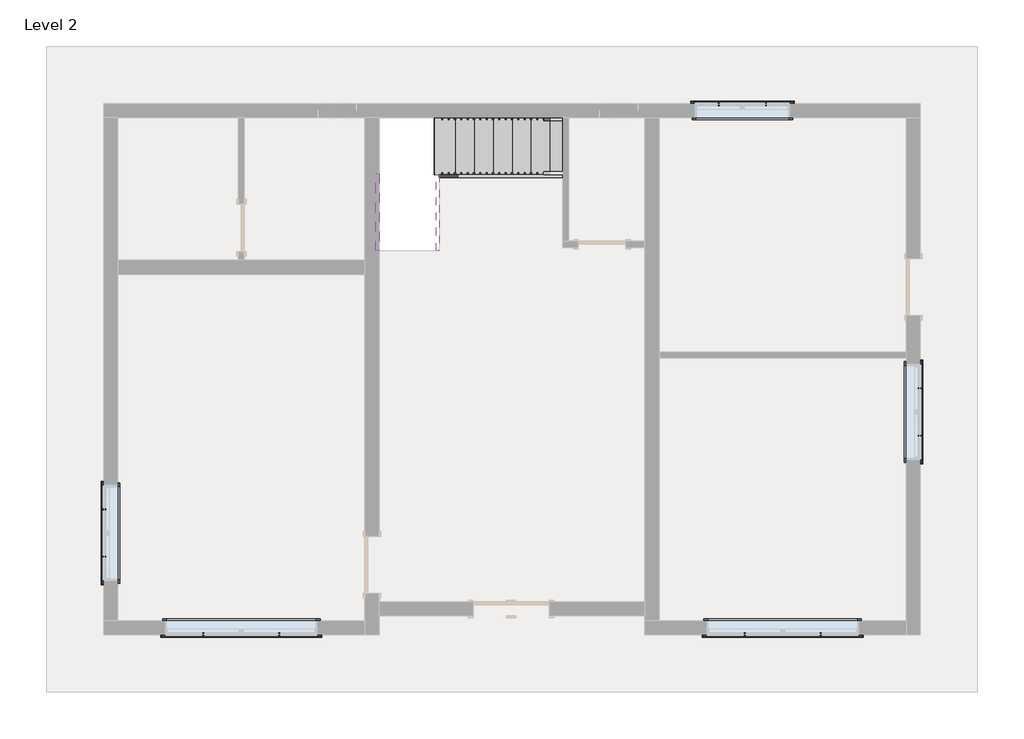
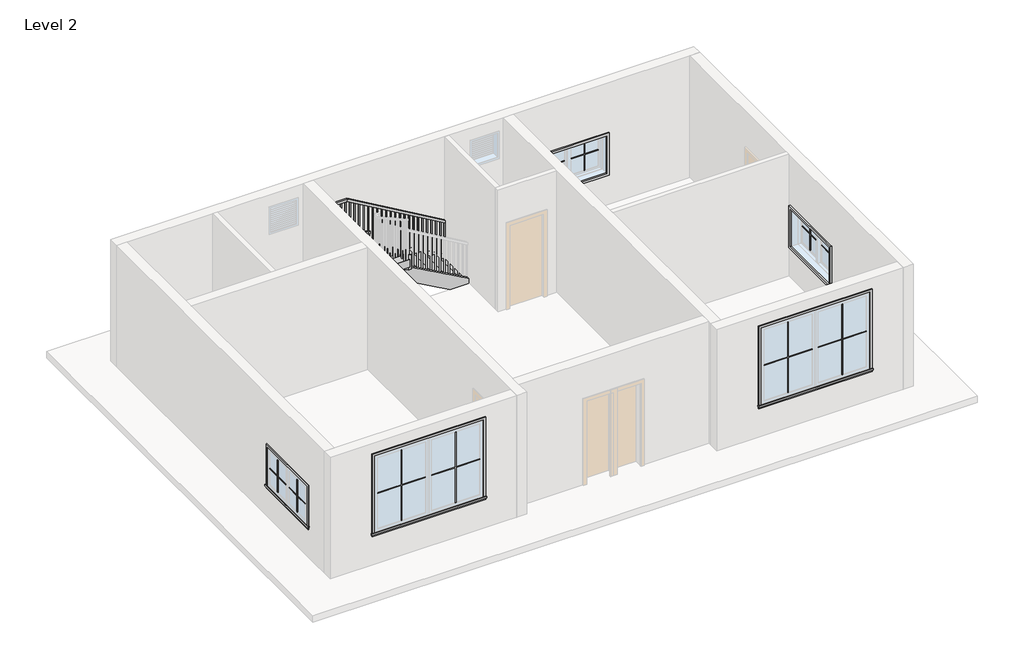
# One storey, part 2 of 2: 20 proxies, 4 members, 1 railing, 1 stair flight.
"""IFC4 building model written with IfcOpenShell, lengths in millimetres."""

from ifc_helpers import new_model, si_unit, frame, origin, place, context, project, spatial, polyline, outline, extrude, faceted_brep, transform, mapped, element, save
from components import muntin_pattern_2x2_muntin_pattern_2x2_9352d081, muntin_pattern_2x2_muntin_pattern_2x2_5c2cbe28, muntin_pattern_2x2_muntin_pattern_2x2_bb8d4d84, muntin_pattern_2x2_muntin_pattern_2x2_d03a1f3c, trim_window_exterior_flat_with_sill_979bde60, trim_window_exterior_flat_with_sill_359ed2ce, trim_window_interior_flat_picture_frame_7883d11b, trim_window_interior_flat_picture_frame_939a8053, stair_flight_cf719367

model = new_model("IFC4")

# Units and contexts
model_context = context("Model", 3, world=origin())
ifc_project = project(units=[si_unit("LENGTHUNIT", "METRE", prefix="MILLI")], contexts=[model_context])

# Site, building, storey
site = spatial("IfcSite", under=ifc_project)
building = spatial("IfcBuilding", under=site)
storey = spatial("IfcBuildingStorey", under=building, Name="Level 2", Elevation=3048.0)

# Proxies
placement = place(None, origin())
muntin_pattern_2x2_muntin_pattern_2x2_shape = muntin_pattern_2x2_muntin_pattern_2x2_9352d081(model_context)
element("IfcBuildingElementProxy", 1, Name="Muntin Pattern_2x2 : Muntin Pattern_2x2", ObjectType="Muntin Pattern_2x2 : Muntin Pattern_2x2", at=placement, inside=storey, context=model_context, shape_type="MappedRepresentation", body=[
    mapped(muntin_pattern_2x2_muntin_pattern_2x2_shape, transform((-7798.9165084, -1764.5743005, 4032.25), x_axis=(0.0, 1.0, 0.0), y_axis=(-1.0, 0.0, 0.0), z_axis=(0.0, 0.0, 1.0))),
])
element("IfcBuildingElementProxy", 2, Name="Muntin Pattern_2x2 : Muntin Pattern_2x2", ObjectType="Muntin Pattern_2x2 : Muntin Pattern_2x2", at=placement, inside=storey, context=model_context, shape_type="MappedRepresentation", body=[
    mapped(muntin_pattern_2x2_muntin_pattern_2x2_shape, transform((5288.4334916, 937.3506995, 4032.25), x_axis=(0.0, -1.0, 0.0), y_axis=(1.0, 0.0, 0.0), z_axis=(0.0, 0.0, 1.0))),
])
element("IfcBuildingElementProxy", 3, Name="Muntin Pattern_2x2 : Muntin Pattern_2x2", ObjectType="Muntin Pattern_2x2 : Muntin Pattern_2x2", at=placement, inside=storey, context=model_context, shape_type="MappedRepresentation", body=[
    mapped(muntin_pattern_2x2_muntin_pattern_2x2_shape, transform((2061.0459916, 5501.4131995, 4032.25), x_axis=(1.0, 0.0, 0.0), y_axis=(0.0, 1.0, 0.0), z_axis=(0.0, 0.0, 1.0))),
])
muntin_pattern_2x2_muntin_pattern_2x2_2_shape = muntin_pattern_2x2_muntin_pattern_2x2_5c2cbe28(model_context)
element("IfcBuildingElementProxy", 4, Name="Muntin Pattern_2x2 : Muntin Pattern_2x2", ObjectType="Muntin Pattern_2x2 : Muntin Pattern_2x2", at=placement, inside=storey, context=model_context, shape_type="MappedRepresentation", body=[
    mapped(muntin_pattern_2x2_muntin_pattern_2x2_2_shape, transform((-7798.9165084, -1005.7493005, 4032.25), x_axis=(0.0, -1.0, 0.0), y_axis=(1.0, 0.0, 0.0), z_axis=(0.0, 0.0, 1.0))),
])
element("IfcBuildingElementProxy", 5, Name="Muntin Pattern_2x2 : Muntin Pattern_2x2", ObjectType="Muntin Pattern_2x2 : Muntin Pattern_2x2", at=placement, inside=storey, context=model_context, shape_type="MappedRepresentation", body=[
    mapped(muntin_pattern_2x2_muntin_pattern_2x2_2_shape, transform((5288.4334916, 178.5256995, 4032.25), x_axis=(0.0, 1.0, 0.0), y_axis=(-1.0, 0.0, 0.0), z_axis=(0.0, 0.0, 1.0))),
])
element("IfcBuildingElementProxy", 6, Name="Muntin Pattern_2x2 : Muntin Pattern_2x2", ObjectType="Muntin Pattern_2x2 : Muntin Pattern_2x2", at=placement, inside=storey, context=model_context, shape_type="MappedRepresentation", body=[
    mapped(muntin_pattern_2x2_muntin_pattern_2x2_2_shape, transform((2819.8709916, 5501.4131995, 4032.25), x_axis=(-1.0, 0.0, 0.0), y_axis=(0.0, -1.0, 0.0), z_axis=(0.0, 0.0, 1.0))),
])
muntin_pattern_2x2_muntin_pattern_2x2_3_shape = muntin_pattern_2x2_muntin_pattern_2x2_bb8d4d84(model_context)
element("IfcBuildingElementProxy", 7, Name="Muntin Pattern_2x2 : Muntin Pattern_2x2", ObjectType="Muntin Pattern_2x2 : Muntin Pattern_2x2", at=placement, inside=storey, context=model_context, shape_type="MappedRepresentation", body=[
    mapped(muntin_pattern_2x2_muntin_pattern_2x2_3_shape, transform((-4990.6290084, -3013.9368005, 4032.25), x_axis=(-1.0, 0.0, 0.0), y_axis=(0.0, -1.0, 0.0), z_axis=(0.0, 0.0, 1.0))),
])
element("IfcBuildingElementProxy", 8, Name="Muntin Pattern_2x2 : Muntin Pattern_2x2", ObjectType="Muntin Pattern_2x2 : Muntin Pattern_2x2", at=placement, inside=storey, context=model_context, shape_type="MappedRepresentation", body=[
    mapped(muntin_pattern_2x2_muntin_pattern_2x2_3_shape, transform((3696.1709916, -3013.9368005, 4032.25), x_axis=(-1.0, 0.0, 0.0), y_axis=(0.0, -1.0, 0.0), z_axis=(0.0, 0.0, 1.0))),
])
muntin_pattern_2x2_muntin_pattern_2x2_4_shape = muntin_pattern_2x2_muntin_pattern_2x2_d03a1f3c(model_context)
element("IfcBuildingElementProxy", 9, Name="Muntin Pattern_2x2 : Muntin Pattern_2x2", ObjectType="Muntin Pattern_2x2 : Muntin Pattern_2x2", at=placement, inside=storey, context=model_context, shape_type="MappedRepresentation", body=[
    mapped(muntin_pattern_2x2_muntin_pattern_2x2_4_shape, transform((-6206.6540084, -3013.9368005, 4032.25), x_axis=(1.0, 0.0, 0.0), y_axis=(0.0, 1.0, 0.0), z_axis=(0.0, 0.0, 1.0))),
])
element("IfcBuildingElementProxy", 10, Name="Muntin Pattern_2x2 : Muntin Pattern_2x2", ObjectType="Muntin Pattern_2x2 : Muntin Pattern_2x2", at=placement, inside=storey, context=model_context, shape_type="MappedRepresentation", body=[
    mapped(muntin_pattern_2x2_muntin_pattern_2x2_4_shape, transform((2480.1459916, -3013.9368005, 4032.25), x_axis=(1.0, 0.0, 0.0), y_axis=(0.0, 1.0, 0.0), z_axis=(0.0, 0.0, 1.0))),
])
trim_window_exterior_flat_with_sill_shape = trim_window_exterior_flat_with_sill_979bde60(model_context)
element("IfcBuildingElementProxy", 11, Name="Trim-Window-Exterior-Flat : with Sill", ObjectType="Trim-Window-Exterior-Flat : with Sill", at=placement, inside=storey, context=model_context, shape_type="MappedRepresentation", body=[
    mapped(trim_window_exterior_flat_with_sill_shape, transform((-7808.4415084, -1385.1618005, 4876.8), x_axis=(0.0, -1.0, 0.0), y_axis=(0.0, 0.0, 1.0), z_axis=(-1.0, 0.0, 0.0))),
])
element("IfcBuildingElementProxy", 12, Name="Trim-Window-Exterior-Flat : with Sill", ObjectType="Trim-Window-Exterior-Flat : with Sill", at=placement, inside=storey, context=model_context, shape_type="MappedRepresentation", body=[
    mapped(trim_window_exterior_flat_with_sill_shape, transform((5297.9584916, 557.9381995, 4876.8), x_axis=(0.0, 1.0, 0.0), y_axis=(0.0, 0.0, 1.0), z_axis=(1.0, 0.0, 0.0))),
])
element("IfcBuildingElementProxy", 13, Name="Trim-Window-Exterior-Flat : with Sill", ObjectType="Trim-Window-Exterior-Flat : with Sill", at=placement, inside=storey, context=model_context, shape_type="MappedRepresentation", body=[
    mapped(trim_window_exterior_flat_with_sill_shape, transform((2440.4584916, 5510.9381995, 4876.8), x_axis=(-1.0, 0.0, 0.0), y_axis=(0.0, 0.0, 1.0), z_axis=(0.0, 1.0, 0.0))),
])
trim_window_exterior_flat_with_sill_2_shape = trim_window_exterior_flat_with_sill_359ed2ce(model_context)
element("IfcBuildingElementProxy", 14, Name="Trim-Window-Exterior-Flat : with Sill", ObjectType="Trim-Window-Exterior-Flat : with Sill", at=placement, inside=storey, context=model_context, shape_type="MappedRepresentation", body=[
    mapped(trim_window_exterior_flat_with_sill_2_shape, transform((-5598.6415084, -3023.4618005, 5791.2), x_axis=(1.0, 0.0, 0.0), y_axis=(0.0, 0.0, 1.0), z_axis=(0.0, -1.0, 0.0))),
])
element("IfcBuildingElementProxy", 15, Name="Trim-Window-Exterior-Flat : with Sill", ObjectType="Trim-Window-Exterior-Flat : with Sill", at=placement, inside=storey, context=model_context, shape_type="MappedRepresentation", body=[
    mapped(trim_window_exterior_flat_with_sill_2_shape, transform((3088.1584916, -3023.4618005, 5791.2), x_axis=(1.0, 0.0, 0.0), y_axis=(0.0, 0.0, 1.0), z_axis=(0.0, -1.0, 0.0))),
])
trim_window_interior_flat_picture_frame_shape = trim_window_interior_flat_picture_frame_7883d11b(model_context)
element("IfcBuildingElementProxy", 16, Name="Trim-Window-Interior-Flat : Picture Frame", ObjectType="Trim-Window-Interior-Flat : Picture Frame", at=placement, inside=storey, context=model_context, shape_type="MappedRepresentation", body=[
    mapped(trim_window_interior_flat_picture_frame_shape, transform((-7579.8415084, -1385.1618005, 4876.8), x_axis=(0.0, 1.0, 0.0), y_axis=(0.0, 0.0, 1.0), z_axis=(1.0, 0.0, 0.0))),
])
element("IfcBuildingElementProxy", 17, Name="Trim-Window-Interior-Flat : Picture Frame", ObjectType="Trim-Window-Interior-Flat : Picture Frame", at=placement, inside=storey, context=model_context, shape_type="MappedRepresentation", body=[
    mapped(trim_window_interior_flat_picture_frame_shape, transform((5069.3584916, 557.9381995, 4876.8), x_axis=(0.0, -1.0, 0.0), y_axis=(0.0, 0.0, 1.0), z_axis=(-1.0, 0.0, 0.0))),
])
element("IfcBuildingElementProxy", 18, Name="Trim-Window-Interior-Flat : Picture Frame", ObjectType="Trim-Window-Interior-Flat : Picture Frame", at=placement, inside=storey, context=model_context, shape_type="MappedRepresentation", body=[
    mapped(trim_window_interior_flat_picture_frame_shape, transform((2440.4584916, 5282.3381995, 4876.8), x_axis=(1.0, 0.0, 0.0), y_axis=(0.0, 0.0, 1.0), z_axis=(0.0, -1.0, 0.0))),
])
trim_window_interior_flat_picture_frame_2_shape = trim_window_interior_flat_picture_frame_939a8053(model_context)
element("IfcBuildingElementProxy", 19, Name="Trim-Window-Interior-Flat : Picture Frame", ObjectType="Trim-Window-Interior-Flat : Picture Frame", at=placement, inside=storey, context=model_context, shape_type="MappedRepresentation", body=[
    mapped(trim_window_interior_flat_picture_frame_2_shape, transform((-5598.6415084, -2794.8618005, 5791.2), x_axis=(-1.0, 0.0, 0.0), y_axis=(0.0, 0.0, 1.0), z_axis=(0.0, 1.0, 0.0))),
])
element("IfcBuildingElementProxy", 20, Name="Trim-Window-Interior-Flat : Picture Frame", ObjectType="Trim-Window-Interior-Flat : Picture Frame", at=placement, inside=storey, context=model_context, shape_type="MappedRepresentation", body=[
    mapped(trim_window_interior_flat_picture_frame_2_shape, transform((3088.1584916, -2794.8618005, 5791.2), x_axis=(-1.0, 0.0, 0.0), y_axis=(0.0, 0.0, 1.0), z_axis=(0.0, 1.0, 0.0))),
])

# Members
element("IfcMember", 21, ObjectType="Stringer - 2\" Width", at=placement, inside=storey, context=model_context, shape_type="SweptSolid", body=[
    extrude(outline(polyline([(3048.0, -442.4415084), (3312.0428392, -442.4415084), (4412.7095059, -2423.6415084), (4064.0308318, -2423.6415084), (3048.0, -594.7860112), (3048.0, -442.4415084)])), frame((0.0, 4317.5146777, 0.0), z_axis=(0.0, 1.0, 0.0), x_axis=(0.0, 0.0, 1.0)), (0.0, 0.0, 1.0), 50.8),
])
element("IfcMember", 22, ObjectType="Stringer - 2\" Width", at=placement, inside=storey, context=model_context, shape_type="SweptSolid", body=[
    extrude(outline(polyline([(4368.3146777, 4610.245537), (4368.3146777, 4261.6006925), (3148.7383287, 4938.8643411), (3148.7383287, 5287.5091856), (4368.3146777, 4610.245537)])), frame((-2474.4415084, 0.0, 0.0), z_axis=(1.0, 0.0, 0.0), x_axis=(0.0, 1.0, 0.0)), (0.0, 0.0, 1.0), 50.8),
])
element("IfcMember", 23, ObjectType="Stringer - 2\" Width", at=placement, inside=storey, context=model_context, shape_type="SweptSolid", body=[
    extrude(outline(polyline([(3048.0, -442.4415084), (3312.0428392, -442.4415084), (4102.6636166, -1865.5589077), (4102.6636166, -2493.1805211), (3048.0, -594.7860112), (3048.0, -442.4415084)])), frame((0.0, 5282.3381995, 0.0), z_axis=(0.0, 1.0, 0.0), x_axis=(0.0, 0.0, 1.0)), (0.0, 0.0, 1.0), 50.8),
])
element("IfcMember", 24, ObjectType="Stringer - 2\" Width", at=placement, inside=storey, context=model_context, shape_type="SweptSolid", body=[
    extrude(outline(polyline([(3758.489521, 4600.253054), (3148.7383287, 4938.8643411), (3148.7383287, 5287.5091856), (4386.3085505, 4600.253054), (3758.489521, 4600.253054)])), frame((-3439.6415084, 0.0, 0.0), z_axis=(1.0, 0.0, 0.0), x_axis=(0.0, 1.0, 0.0)), (0.0, 0.0, 1.0), 50.8),
])

# Railing
element("IfcRailing", 25, ObjectType="Handrail - Rectangular", at=placement, inside=storey, context=model_context, shape_type="SolidModel", body=[
    faceted_brep([(-442.4415084, 5231.5381995, 4131.7333333), (-442.4415084, 5231.5381995, 4072.9219871), (-442.4415084, 5282.3381995, 4072.9219871), (-442.4415084, 5282.3381995, 4131.7333333), (-2641.0608886, 5231.5381995, 5414.2613051), (-2654.794625, 5231.5381995, 5363.4613051), (-2654.794625, 5282.3381995, 5363.4613051), (-2641.0608886, 5282.3381995, 5414.2613051), (-3338.0415084, 5231.5381995, 5414.2613051), (-3338.0415084, 5231.5381995, 5363.4613051), (-3388.8415084, 5282.3381995, 5363.4613051), (-3388.8415084, 5282.3381995, 5414.2613051), (-3338.0415084, 4498.2044111, 5414.2613051), (-3338.0415084, 4485.04436, 5363.4613051), (-3388.8415084, 4485.04436, 5363.4613051), (-3388.8415084, 4498.2044111, 5414.2613051), (-3338.0415084, 3148.7383287, 6163.7333333), (-3388.8415084, 3148.7383287, 6163.7333333), (-3388.8415084, 3148.7383287, 6105.62445), (-3338.0415084, 3148.7383287, 6105.62445)], [[[0, 1, 2, 3]], [[1, 0, 4, 5]], [[2, 1, 5, 6]], [[3, 2, 6, 7]], [[0, 3, 7, 4]], [[5, 4, 8, 9]], [[6, 5, 9, 10]], [[7, 6, 10, 11]], [[4, 7, 11, 8]], [[9, 8, 12, 13]], [[10, 9, 13, 14]], [[11, 10, 14, 15]], [[8, 11, 15, 12]], [[16, 17, 18, 19]], [[13, 12, 16, 19]], [[14, 13, 19, 18]], [[15, 14, 18, 17]], [[12, 15, 17, 16]]]),
    extrude(outline(polyline([(3215.4131995, 6068.5942858), (3234.4631995, 6058.0142183), (3234.4631995, 5080.0), (3215.4131995, 5080.0), (3215.4131995, 6068.5942858)])), frame((-3372.9665084, 0.0, 0.0), z_axis=(1.0, 0.0, 0.0), x_axis=(0.0, 1.0, 0.0)), (0.0, 0.0, 1.0), 19.05),
    extrude(outline(polyline([(3317.0131995, 6012.3240232), (3336.0631995, 6001.7439558), (3336.0631995, 5080.0), (3317.0131995, 5080.0), (3317.0131995, 6012.3240232)])), frame((-3372.9665084, 0.0, 0.0), z_axis=(1.0, 0.0, 0.0), x_axis=(0.0, 1.0, 0.0)), (0.0, 0.0, 1.0), 19.05),
    extrude(outline(polyline([(3418.6131995, 5955.8969969), (3437.6631995, 5945.3169295), (3437.6631995, 5080.0), (3418.6131995, 5080.0), (3418.6131995, 5955.8969969)])), frame((-3372.9665084, 0.0, 0.0), z_axis=(1.0, 0.0, 0.0), x_axis=(0.0, 1.0, 0.0)), (0.0, 0.0, 1.0), 19.05),
    extrude(outline(polyline([(3520.2131995, 5899.4699707), (3539.2631995, 5888.8899033), (3539.2631995, 4910.6666667), (3520.2131995, 4910.6666667), (3520.2131995, 5899.4699707)])), frame((-3372.9665084, 0.0, 0.0), z_axis=(1.0, 0.0, 0.0), x_axis=(0.0, 1.0, 0.0)), (0.0, 0.0, 1.0), 19.05),
    extrude(outline(polyline([(3621.8131995, 5842.9906899), (3640.8631995, 5832.4106224), (3640.8631995, 4910.6666667), (3621.8131995, 4910.6666667), (3621.8131995, 5842.9906899)])), frame((-3372.9665084, 0.0, 0.0), z_axis=(1.0, 0.0, 0.0), x_axis=(0.0, 1.0, 0.0)), (0.0, 0.0, 1.0), 19.05),
    extrude(outline(polyline([(3723.4131995, 5786.5636636), (3742.4631995, 5775.9835962), (3742.4631995, 4910.6666667), (3723.4131995, 4910.6666667), (3723.4131995, 5786.5636636)])), frame((-3372.9665084, 0.0, 0.0), z_axis=(1.0, 0.0, 0.0), x_axis=(0.0, 1.0, 0.0)), (0.0, 0.0, 1.0), 19.05),
    extrude(outline(polyline([(3825.0131995, 5730.1366374), (3844.0631995, 5719.5565699), (3844.0631995, 4741.3333333), (3825.0131995, 4741.3333333), (3825.0131995, 5730.1366374)])), frame((-3372.9665084, 0.0, 0.0), z_axis=(1.0, 0.0, 0.0), x_axis=(0.0, 1.0, 0.0)), (0.0, 0.0, 1.0), 19.05),
    extrude(outline(polyline([(3926.6131995, 5673.6573565), (3945.6631995, 5663.0772891), (3945.6631995, 4741.3333333), (3926.6131995, 4741.3333333), (3926.6131995, 5673.6573565)])), frame((-3372.9665084, 0.0, 0.0), z_axis=(1.0, 0.0, 0.0), x_axis=(0.0, 1.0, 0.0)), (0.0, 0.0, 1.0), 19.05),
    extrude(outline(polyline([(4028.2131995, 5617.2303303), (4047.2631995, 5606.6502629), (4047.2631995, 4741.3333333), (4028.2131995, 4741.3333333), (4028.2131995, 5617.2303303)])), frame((-3372.9665084, 0.0, 0.0), z_axis=(1.0, 0.0, 0.0), x_axis=(0.0, 1.0, 0.0)), (0.0, 0.0, 1.0), 19.05),
    extrude(outline(polyline([(4129.8131995, 5560.803304), (4148.8631995, 5550.2232366), (4148.8631995, 4572.0), (4129.8131995, 4572.0), (4129.8131995, 5560.803304)])), frame((-3372.9665084, 0.0, 0.0), z_axis=(1.0, 0.0, 0.0), x_axis=(0.0, 1.0, 0.0)), (0.0, 0.0, 1.0), 19.05),
    extrude(outline(polyline([(4231.4131995, 5504.3240232), (4250.4631995, 5493.7439558), (4250.4631995, 4572.0), (4231.4131995, 4572.0), (4231.4131995, 5504.3240232)])), frame((-3372.9665084, 0.0, 0.0), z_axis=(1.0, 0.0, 0.0), x_axis=(0.0, 1.0, 0.0)), (0.0, 0.0, 1.0), 19.05),
    extrude(outline(polyline([(4333.0131995, 5447.8969969), (4352.0631995, 5437.3169295), (4352.0631995, 4572.0), (4333.0131995, 4572.0), (4333.0131995, 5447.8969969)])), frame((-3372.9665084, 0.0, 0.0), z_axis=(1.0, 0.0, 0.0), x_axis=(0.0, 1.0, 0.0)), (0.0, 0.0, 1.0), 19.05),
    extrude(outline(polyline([(4434.6131995, 5391.4699707), (4453.6631995, 5380.8899033), (4453.6631995, 4402.6666667), (4434.6131995, 4402.6666667), (4434.6131995, 5391.4699707)])), frame((-3372.9665084, 0.0, 0.0), z_axis=(1.0, 0.0, 0.0), x_axis=(0.0, 1.0, 0.0)), (0.0, 0.0, 1.0), 19.05),
    extrude(outline(polyline([(-3372.9665084, 4555.2631995), (-3353.9165084, 4555.2631995), (-3353.9165084, 4536.2131995), (-3372.9665084, 4536.2131995), (-3372.9665084, 4555.2631995)])), frame((0.0, 0.0, 4402.6666667), z_axis=(0.0, 0.0, 1.0), x_axis=(1.0, 0.0, 0.0)), (0.0, 0.0, 1.0), 960.7946385),
    extrude(outline(polyline([(-3372.9665084, 4656.8631995), (-3353.9165084, 4656.8631995), (-3353.9165084, 4637.8131995), (-3372.9665084, 4637.8131995), (-3372.9665084, 4656.8631995)])), frame((0.0, 0.0, 4402.6666667), z_axis=(0.0, 0.0, 1.0), x_axis=(1.0, 0.0, 0.0)), (0.0, 0.0, 1.0), 960.7946385),
    extrude(outline(polyline([(-3372.9665084, 4758.4631995), (-3353.9165084, 4758.4631995), (-3353.9165084, 4739.4131995), (-3372.9665084, 4739.4131995), (-3372.9665084, 4758.4631995)])), frame((0.0, 0.0, 4402.6666667), z_axis=(0.0, 0.0, 1.0), x_axis=(1.0, 0.0, 0.0)), (0.0, 0.0, 1.0), 960.7946385),
    extrude(outline(polyline([(-3372.9665084, 4860.0631995), (-3353.9165084, 4860.0631995), (-3353.9165084, 4841.0131995), (-3372.9665084, 4841.0131995), (-3372.9665084, 4860.0631995)])), frame((0.0, 0.0, 4402.6666667), z_axis=(0.0, 0.0, 1.0), x_axis=(1.0, 0.0, 0.0)), (0.0, 0.0, 1.0), 960.7946385),
    extrude(outline(polyline([(-3372.9665084, 4961.6631995), (-3353.9165084, 4961.6631995), (-3353.9165084, 4942.6131995), (-3372.9665084, 4942.6131995), (-3372.9665084, 4961.6631995)])), frame((0.0, 0.0, 4402.6666667), z_axis=(0.0, 0.0, 1.0), x_axis=(1.0, 0.0, 0.0)), (0.0, 0.0, 1.0), 960.7946385),
    extrude(outline(polyline([(-3372.9665084, 5063.2631995), (-3353.9165084, 5063.2631995), (-3353.9165084, 5044.2131995), (-3372.9665084, 5044.2131995), (-3372.9665084, 5063.2631995)])), frame((0.0, 0.0, 4402.6666667), z_axis=(0.0, 0.0, 1.0), x_axis=(1.0, 0.0, 0.0)), (0.0, 0.0, 1.0), 960.7946385),
    extrude(outline(polyline([(-3372.9665084, 5164.8631995), (-3353.9165084, 5164.8631995), (-3353.9165084, 5145.8131995), (-3372.9665084, 5145.8131995), (-3372.9665084, 5164.8631995)])), frame((0.0, 0.0, 4402.6666667), z_axis=(0.0, 0.0, 1.0), x_axis=(1.0, 0.0, 0.0)), (0.0, 0.0, 1.0), 960.7946385),
    extrude(outline(polyline([(-3277.7165084, 5266.4631995), (-3277.7165084, 5247.4131995), (-3296.7665084, 5247.4131995), (-3296.7665084, 5266.4631995), (-3277.7165084, 5266.4631995)])), frame((0.0, 0.0, 4402.6666667), z_axis=(0.0, 0.0, 1.0), x_axis=(1.0, 0.0, 0.0)), (0.0, 0.0, 1.0), 960.7946385),
    extrude(outline(polyline([(-3176.1165084, 5266.4631995), (-3176.1165084, 5247.4131995), (-3195.1665084, 5247.4131995), (-3195.1665084, 5266.4631995), (-3176.1165084, 5266.4631995)])), frame((0.0, 0.0, 4402.6666667), z_axis=(0.0, 0.0, 1.0), x_axis=(1.0, 0.0, 0.0)), (0.0, 0.0, 1.0), 960.7946385),
    extrude(outline(polyline([(-3074.5165084, 5266.4631995), (-3074.5165084, 5247.4131995), (-3093.5665084, 5247.4131995), (-3093.5665084, 5266.4631995), (-3074.5165084, 5266.4631995)])), frame((0.0, 0.0, 4402.6666667), z_axis=(0.0, 0.0, 1.0), x_axis=(1.0, 0.0, 0.0)), (0.0, 0.0, 1.0), 960.7946385),
    extrude(outline(polyline([(-2972.9165084, 5266.4631995), (-2972.9165084, 5247.4131995), (-2991.9665084, 5247.4131995), (-2991.9665084, 5266.4631995), (-2972.9165084, 5266.4631995)])), frame((0.0, 0.0, 4402.6666667), z_axis=(0.0, 0.0, 1.0), x_axis=(1.0, 0.0, 0.0)), (0.0, 0.0, 1.0), 960.7946385),
    extrude(outline(polyline([(-2871.3165084, 5266.4631995), (-2871.3165084, 5247.4131995), (-2890.3665084, 5247.4131995), (-2890.3665084, 5266.4631995), (-2871.3165084, 5266.4631995)])), frame((0.0, 0.0, 4402.6666667), z_axis=(0.0, 0.0, 1.0), x_axis=(1.0, 0.0, 0.0)), (0.0, 0.0, 1.0), 960.7946385),
    extrude(outline(polyline([(-2769.7165084, 5266.4631995), (-2769.7165084, 5247.4131995), (-2788.7665084, 5247.4131995), (-2788.7665084, 5266.4631995), (-2769.7165084, 5266.4631995)])), frame((0.0, 0.0, 4402.6666667), z_axis=(0.0, 0.0, 1.0), x_axis=(1.0, 0.0, 0.0)), (0.0, 0.0, 1.0), 960.7946385),
    extrude(outline(polyline([(-2668.1165084, 5266.4631995), (-2668.1165084, 5247.4131995), (-2687.1665084, 5247.4131995), (-2687.1665084, 5266.4631995), (-2668.1165084, 5266.4631995)])), frame((0.0, 0.0, 4402.6666667), z_axis=(0.0, 0.0, 1.0), x_axis=(1.0, 0.0, 0.0)), (0.0, 0.0, 1.0), 960.7946385),
    extrude(outline(polyline([(5311.9657371, -2566.5165084), (5323.0782371, -2585.5665084), (4402.6666667, -2585.5665084), (4402.6666667, -2566.5165084), (5311.9657371, -2566.5165084)])), frame((0.0, 5247.4131995, 0.0), z_axis=(0.0, 1.0, 0.0), x_axis=(0.0, 0.0, 1.0)), (0.0, 0.0, 1.0), 19.05),
    extrude(outline(polyline([(5252.6990704, -2464.9165084), (5263.8115704, -2483.9665084), (4402.6666667, -2483.9665084), (4402.6666667, -2464.9165084), (5252.6990704, -2464.9165084)])), frame((0.0, 5247.4131995, 0.0), z_axis=(0.0, 1.0, 0.0), x_axis=(0.0, 0.0, 1.0)), (0.0, 0.0, 1.0), 19.05),
    extrude(outline(polyline([(5193.4324038, -2363.3165084), (5204.5449038, -2382.3665084), (4233.3333333, -2382.3665084), (4233.3333333, -2363.3165084), (5193.4324038, -2363.3165084)])), frame((0.0, 5247.4131995, 0.0), z_axis=(0.0, 1.0, 0.0), x_axis=(0.0, 0.0, 1.0)), (0.0, 0.0, 1.0), 19.05),
    extrude(outline(polyline([(5134.1657371, -2261.7165084), (5145.2782371, -2280.7665084), (4233.3333333, -2280.7665084), (4233.3333333, -2261.7165084), (5134.1657371, -2261.7165084)])), frame((0.0, 5247.4131995, 0.0), z_axis=(0.0, 1.0, 0.0), x_axis=(0.0, 0.0, 1.0)), (0.0, 0.0, 1.0), 19.05),
    extrude(outline(polyline([(5074.8990704, -2160.1165084), (5086.0115704, -2179.1665084), (4233.3333333, -2179.1665084), (4233.3333333, -2160.1165084), (5074.8990704, -2160.1165084)])), frame((0.0, 5247.4131995, 0.0), z_axis=(0.0, 1.0, 0.0), x_axis=(0.0, 0.0, 1.0)), (0.0, 0.0, 1.0), 19.05),
    extrude(outline(polyline([(5015.6324038, -2058.5165084), (5026.7449038, -2077.5665084), (4064.0, -2077.5665084), (4064.0, -2058.5165084), (5015.6324038, -2058.5165084)])), frame((0.0, 5247.4131995, 0.0), z_axis=(0.0, 1.0, 0.0), x_axis=(0.0, 0.0, 1.0)), (0.0, 0.0, 1.0), 19.05),
    extrude(outline(polyline([(4956.3657371, -1956.9165084), (4967.4782371, -1975.9665084), (4064.0, -1975.9665084), (4064.0, -1956.9165084), (4956.3657371, -1956.9165084)])), frame((0.0, 5247.4131995, 0.0), z_axis=(0.0, 1.0, 0.0), x_axis=(0.0, 0.0, 1.0)), (0.0, 0.0, 1.0), 19.05),
    extrude(outline(polyline([(4897.0990704, -1855.3165084), (4908.2115704, -1874.3665084), (4064.0, -1874.3665084), (4064.0, -1855.3165084), (4897.0990704, -1855.3165084)])), frame((0.0, 5247.4131995, 0.0), z_axis=(0.0, 1.0, 0.0), x_axis=(0.0, 0.0, 1.0)), (0.0, 0.0, 1.0), 19.05),
    extrude(outline(polyline([(4837.8324038, -1753.7165084), (4848.9449038, -1772.7665084), (3894.6666667, -1772.7665084), (3894.6666667, -1753.7165084), (4837.8324038, -1753.7165084)])), frame((0.0, 5247.4131995, 0.0), z_axis=(0.0, 1.0, 0.0), x_axis=(0.0, 0.0, 1.0)), (0.0, 0.0, 1.0), 19.05),
    extrude(outline(polyline([(4778.5657371, -1652.1165084), (4789.6782371, -1671.1665084), (3894.6666667, -1671.1665084), (3894.6666667, -1652.1165084), (4778.5657371, -1652.1165084)])), frame((0.0, 5247.4131995, 0.0), z_axis=(0.0, 1.0, 0.0), x_axis=(0.0, 0.0, 1.0)), (0.0, 0.0, 1.0), 19.05),
    extrude(outline(polyline([(4719.2990704, -1550.5165084), (4730.4115704, -1569.5665084), (3894.6666667, -1569.5665084), (3894.6666667, -1550.5165084), (4719.2990704, -1550.5165084)])), frame((0.0, 5247.4131995, 0.0), z_axis=(0.0, 1.0, 0.0), x_axis=(0.0, 0.0, 1.0)), (0.0, 0.0, 1.0), 19.05),
    extrude(outline(polyline([(4660.0324038, -1448.9165084), (4671.1449038, -1467.9665084), (3725.3333333, -1467.9665084), (3725.3333333, -1448.9165084), (4660.0324038, -1448.9165084)])), frame((0.0, 5247.4131995, 0.0), z_axis=(0.0, 1.0, 0.0), x_axis=(0.0, 0.0, 1.0)), (0.0, 0.0, 1.0), 19.05),
    extrude(outline(polyline([(4600.7657371, -1347.3165084), (4611.8782371, -1366.3665084), (3725.3333333, -1366.3665084), (3725.3333333, -1347.3165084), (4600.7657371, -1347.3165084)])), frame((0.0, 5247.4131995, 0.0), z_axis=(0.0, 1.0, 0.0), x_axis=(0.0, 0.0, 1.0)), (0.0, 0.0, 1.0), 19.05),
    extrude(outline(polyline([(4541.4990704, -1245.7165084), (4552.6115704, -1264.7665084), (3725.3333333, -1264.7665084), (3725.3333333, -1245.7165084), (4541.4990704, -1245.7165084)])), frame((0.0, 5247.4131995, 0.0), z_axis=(0.0, 1.0, 0.0), x_axis=(0.0, 0.0, 1.0)), (0.0, 0.0, 1.0), 19.05),
    extrude(outline(polyline([(4482.2324038, -1144.1165084), (4493.3449038, -1163.1665084), (3556.0, -1163.1665084), (3556.0, -1144.1165084), (4482.2324038, -1144.1165084)])), frame((0.0, 5247.4131995, 0.0), z_axis=(0.0, 1.0, 0.0), x_axis=(0.0, 0.0, 1.0)), (0.0, 0.0, 1.0), 19.05),
    extrude(outline(polyline([(4422.9657371, -1042.5165084), (4434.0782371, -1061.5665084), (3556.0, -1061.5665084), (3556.0, -1042.5165084), (4422.9657371, -1042.5165084)])), frame((0.0, 5247.4131995, 0.0), z_axis=(0.0, 1.0, 0.0), x_axis=(0.0, 0.0, 1.0)), (0.0, 0.0, 1.0), 19.05),
    extrude(outline(polyline([(4363.6990704, -940.9165084), (4374.8115704, -959.9665084), (3556.0, -959.9665084), (3556.0, -940.9165084), (4363.6990704, -940.9165084)])), frame((0.0, 5247.4131995, 0.0), z_axis=(0.0, 1.0, 0.0), x_axis=(0.0, 0.0, 1.0)), (0.0, 0.0, 1.0), 19.05),
    extrude(outline(polyline([(4304.4324038, -839.3165084), (4315.5449038, -858.3665084), (3386.6666667, -858.3665084), (3386.6666667, -839.3165084), (4304.4324038, -839.3165084)])), frame((0.0, 5247.4131995, 0.0), z_axis=(0.0, 1.0, 0.0), x_axis=(0.0, 0.0, 1.0)), (0.0, 0.0, 1.0), 19.05),
    extrude(outline(polyline([(4245.1657371, -737.7165084), (4256.2782371, -756.7665084), (3386.6666667, -756.7665084), (3386.6666667, -737.7165084), (4245.1657371, -737.7165084)])), frame((0.0, 5247.4131995, 0.0), z_axis=(0.0, 1.0, 0.0), x_axis=(0.0, 0.0, 1.0)), (0.0, 0.0, 1.0), 19.05),
    extrude(outline(polyline([(4185.8990704, -636.1165084), (4197.0115704, -655.1665084), (3386.6666667, -655.1665084), (3386.6666667, -636.1165084), (4185.8990704, -636.1165084)])), frame((0.0, 5247.4131995, 0.0), z_axis=(0.0, 1.0, 0.0), x_axis=(0.0, 0.0, 1.0)), (0.0, 0.0, 1.0), 19.05),
    extrude(outline(polyline([(4126.6324038, -534.5165084), (4137.7449038, -553.5665084), (3217.3333333, -553.5665084), (3217.3333333, -534.5165084), (4126.6324038, -534.5165084)])), frame((0.0, 5247.4131995, 0.0), z_axis=(0.0, 1.0, 0.0), x_axis=(0.0, 0.0, 1.0)), (0.0, 0.0, 1.0), 19.05),
    extrude(outline(polyline([(-3353.9165084, 5266.4631995), (-3353.9165084, 5247.4131995), (-3372.9665084, 5247.4131995), (-3372.9665084, 5266.4631995), (-3353.9165084, 5266.4631995)])), frame((0.0, 0.0, 4402.6666667), z_axis=(0.0, 0.0, 1.0), x_axis=(1.0, 0.0, 0.0)), (0.0, 0.0, 1.0), 960.7946385),
    extrude(outline(polyline([(3148.7383287, 6105.62445), (3167.7883287, 6095.0443826), (3167.7883287, 5080.0), (3148.7383287, 5080.0), (3148.7383287, 6105.62445)])), frame((-3372.9665084, 0.0, 0.0), z_axis=(1.0, 0.0, 0.0), x_axis=(0.0, 1.0, 0.0)), (0.0, 0.0, 1.0), 19.05),
    extrude(outline(polyline([(4072.9219871, -442.4415084), (4084.0344871, -461.4915084), (3217.3333333, -461.4915084), (3217.3333333, -442.4415084), (4072.9219871, -442.4415084)])), frame((0.0, 5247.4131995, 0.0), z_axis=(0.0, 1.0, 0.0), x_axis=(0.0, 0.0, 1.0)), (0.0, 0.0, 1.0), 19.05),
])

# Stair flight
stair_flight_shape = stair_flight_cf719367(model_context)
element("IfcStairFlight", 26, ObjectType="2\" Tread 1\" Nosing 1/4\" Riser", at=placement, inside=storey, context=model_context, shape_type="MappedRepresentation", body=[
    mapped(stair_flight_shape, transform((0.0, 0.0, 0.0), x_axis=(1.0, 0.0, 0.0), y_axis=(0.0, 1.0, 0.0), z_axis=(0.0, 0.0, 1.0))),
])

save(model, "model.ifc")

# Revit data of these elements
# Type "Muntin Pattern_2x2 : Muntin Pattern_2x2"
#   Width [instance default] = 4' - 0"
#   Thickness = 0' - 0 1/2"
#   Height [instance default] = 4' - 0"
#   Distance = 0' - 0 3/4"
#   Interior Material [instance default] = none
#   Exterior Material [instance default] = none
#   Default Elevation = 0
# Type "Trim-Window-Exterior-Flat : with Sill"
#   Trim Width = 0' - 2 1/4"
#   Trim Thickness_Picture Frame = 0' - 1 1/4"
#   Trim Thickness_with Sill = 0' - 0 3/4"
#   Sill Thickness = 0' - 1 1/4"
#   Opening Width [instance default] = 2' - 0"
#   Opening Height [instance default] = 3' - 0"
#   Default Elevation = 4' - 0"
#   Sill = yes
#   Picture Frame = no
#   Trim Material [instance default] = none
# Type "Trim-Window-Interior-Flat : Picture Frame"
#   Trim Thickness_Picture Frame = 0' - 1 1/4"
#   Trim Width = 0' - 2 1/4"
#   Trim Thickness_with Sill = 0' - 0 3/4"
#   Sill Thickness = 0' - 1 1/4"
#   Opening Width [instance default] = 2' - 0"
#   Opening Height [instance default] = 3' - 0"
#   Default Elevation = 4' - 0"
#   Sill = no
#   Picture Frame = yes
#   Trim Material [instance default] = none
# Type "Handrail - Rectangular"
#   Assembly Code = "C2010400"
#   built-in parameter 1008612 = 0.0416667 (stored number, unit not read)
#   built-in parameter 1008611 = 0.0416667 (stored number, unit not read)
#   built-in parameter 1008609 = 0.333333 (stored number, unit not read)
#   built-in parameter 1008604 = 0.166667 (stored number, unit not read)
#   built-in parameter 1008603 = 0.166667 (stored number, unit not read)
#   Railing Height = 3' - 0"
#   built-in parameter 1008630 = 2
#   built-in parameter 1008610 = 2
#   built-in parameter 1008618 = Baluster - Square : 3/4"
# Elements 1, 2, 3, 4, 5, 6 (IfcBuildingElementProxy, "Muntin Pattern_2x2 : Muntin Pattern_2x2")
#   Width = 2' - 0 5/8"
#   Height = 2' - 6 1/2"
#   Interior Material = Wood - Stained
#   Exterior Material = Clad - White
#   Phase Created = New Construction
#   Materials on its faces: "Clad - White", "Wood - Stained"
# Elements 7, 8, 9, 10 (IfcBuildingElementProxy, "Muntin Pattern_2x2 : Muntin Pattern_2x2")
#   Width = 3' - 6 5/8"
#   Height = 5' - 6 1/2"
#   Interior Material = Wood - Stained
#   Exterior Material = Clad - White
#   Phase Created = New Construction
#   Materials on its faces: "Clad - White", "Wood - Stained"
# Elements 11, 12, 13 (IfcBuildingElementProxy, "Trim-Window-Exterior-Flat : with Sill")
#   Opening Width = 5' - 0"
#   Opening Height = 3' - 0"
#   Trim Material = Clad - White
#   Phase Created = New Construction
#   Materials on its faces: "Clad - White"
# Elements 14, 15 (IfcBuildingElementProxy, "Trim-Window-Exterior-Flat : with Sill")
#   Opening Width = 8' - 0"
#   Opening Height = 6' - 0"
#   Trim Material = Clad - White
#   Phase Created = New Construction
#   Materials on its faces: "Clad - White"
# Elements 16, 17, 18 (IfcBuildingElementProxy, "Trim-Window-Interior-Flat : Picture Frame")
#   Opening Width = 5' - 0"
#   Opening Height = 3' - 0"
#   Trim Material = Wood - Stained
#   Phase Created = New Construction
#   Materials on its faces: "Wood - Stained"
# Elements 19, 20 (IfcBuildingElementProxy, "Trim-Window-Interior-Flat : Picture Frame")
#   Opening Width = 8' - 0"
#   Opening Height = 6' - 0"
#   Trim Material = Wood - Stained
#   Phase Created = New Construction
#   Materials on its faces: "Wood - Stained"
# Elements 21, 22, 23, 24 (IfcMember, "Stringer - 2\" Width")
#   Phase Created = New Construction
# Element 25 (IfcRailing, "Handrail - Rectangular")
#   Phase Created = New Construction
# Element 26 (IfcStairFlight, "2\" Tread 1\" Nosing 1/4\" Riser")
#   Phase Created = New Construction
# Materials
#   "Clad - White": class "Wood", colour RGB 242 242 238, transparency 0, Cost = 0
#   "Wood - Stained": class "Wood", colour RGB 224 178 126, transparency 0, Cost = 0
